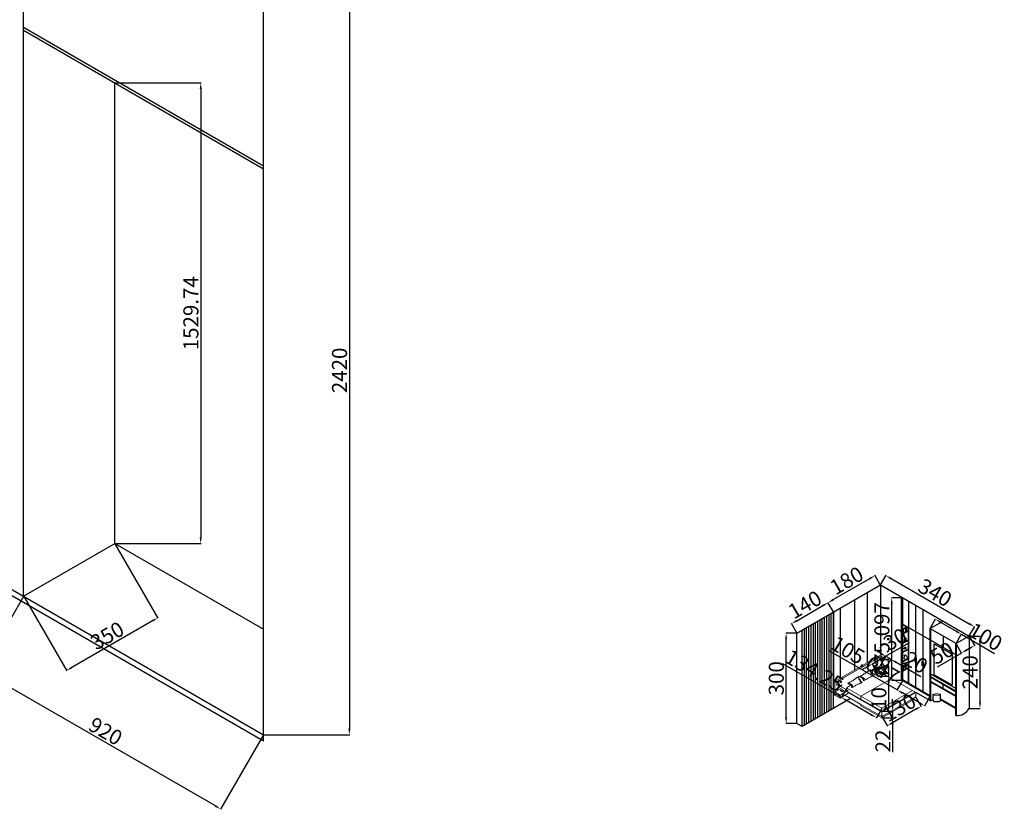
# Model space of a CAD drawing. Units: centimetres. Extents: x 209356 to 217348, y 253987 to 259034.
# Tile 6 of 7: x 214078 to 217348, y 254619 to 257241. Entities that reach past the tile are written whole.
import ezdxf

# ---------------------------------------------------------------- set-up
doc = ezdxf.new("R2010")
doc.units = ezdxf.units.CM
for name, color, linetype, lineweight in [('A-ANNO-DIMS', 2, 'Continuous', 18), ('A-ELEV', 7, 'Continuous', 25), ('A-FURN', 8, 'Continuous', 18)]:
    doc.layers.add(name, color=color, linetype=linetype, lineweight=lineweight)
doc.styles.get("Standard").update_dxf_attribs({"font": 'arial.ttf'})
doc.dimstyles.new('ISO-25', dxfattribs={"dimtxt": 50, "dimasz": 20, "dimexe": 1.25, "dimexo": 0.625, "dimtad": 1, "dimdec": 1, "dimtxsty": 'Standard', "dimcen": 2.5, "dimadec": 0, "dimazin": 0, "dimtfac": 1, "dimtdec": 1, "dimtmove": 0, "dimatfit": 3, "dimfxl": 1, "dimarcsym": 0})

# ---------------------------------------------------------------- blocks, each defined once
blk = doc.blocks.new('BED')
for p, q in [((217490, 254381.4), (217645.9, 254471.4)), ((217494.4, 254378.9), (217650.2, 254468.9)), ((217650.2, 254468.9), (217645.9, 254471.4)), ((217650.2, 254468.9), (217650.2, 254433.8)), ((217619.9, 254421.3), (217645.9, 254436.3)), ((217637.2, 254411.3), (217619.9, 254421.3)), ((217619.9, 254421.3), (217619.9, 254411.3)), ((217637.2, 254401.3), (217619.9, 254411.3)), ((217623.4, 254433.4), (217628.8, 254436.6)), ((217623.4, 254430.2), (217623.4, 254433.4)), ((217623.4, 254430.2), (217628.8, 254433.4)), ((217628.8, 254436.6), (217628.8, 254433.4)), ((217630.5, 254437.7), (217636, 254440.8)), ((217630.5, 254434.5), (217630.5, 254437.7)), ((217630.5, 254434.5), (217636, 254437.6)), ((217631.5, 254423.4), (217637.4, 254426.8)), ((217638.6, 254420.1), (217631.5, 254423.4)), ((217636, 254440.8), (217636, 254437.6)), ((217637.2, 254411.3), (217663.2, 254426.3)), ((217663.2, 254416.3), (217637.2, 254401.3)), ((217637.2, 254411.3), (217637.2, 254401.3)), ((217637.4, 254426.8), (217643.8, 254423.1)), ((217643.8, 254423.1), (217638.6, 254420.1)), ((217642.5, 254427.6), (217641.6, 254424.4)), ((217642.4, 254423.9), (217645.6, 254425.8)), ((217645.6, 254425.8), (217642.5, 254427.6)), ((217645.9, 254436.3), (217663.2, 254426.3)), ((217763, 254347.7), (217653.8, 254410.8)), ((217663.2, 254426.3), (217663.2, 254416.3)), ((217490, 254341.4), (217490, 254381.4)), ((217490, 254381.4), (217494.4, 254378.9)), ((217494.4, 254378.9), (217494.4, 254338.9)), ((217505.5, 254383.3), (217501.1, 254380.8)), ((217501.1, 254380.8), (217501.1, 254370.1)), ((217505.5, 254372.6), (217505.5, 254383.3)), ((217683.4, 254393.7), (217581.2, 254334.7)), ((217494.4, 254348.9), (217520.3, 254363.9)), ((217511.7, 254338.9), (217494.4, 254348.9)), ((217501.1, 254370.1), (217505.5, 254372.6)), ((217504.8, 254365), (217510.2, 254368.1)), ((217504.8, 254361.8), (217504.8, 254365)), ((217504.8, 254361.8), (217510.2, 254364.9)), ((217510.2, 254368.1), (217510.2, 254364.9)), ((217511.7, 254338.9), (217537.7, 254353.9)), ((217511.9, 254369.2), (217517.4, 254372.4)), ((217511.9, 254366), (217511.9, 254369.2)), ((217511.9, 254366), (217517.4, 254369.2)), ((217512.1, 254354), (217517.6, 254357.2)), ((217519.3, 254349.8), (217512.1, 254354)), ((217513.4, 254354), (217513.7, 254354.1)), ((217519.4, 254350.5), (217513.4, 254354)), ((217513.7, 254354.1), (217519.6, 254350.7)), ((217517.4, 254372.4), (217517.4, 254369.2)), ((217517.6, 254357.2), (217524.8, 254353)), ((217524.8, 254353), (217519.3, 254349.8)), ((217519.6, 254350.7), (217519.4, 254350.5)), ((217520.3, 254363.9), (217537.7, 254353.9)), ((217650.5, 254294.7), (217534.2, 254361.9)), ((217534.2, 254361.9), (217534.2, 254355.9)), ((217537.7, 254353.9), (217537.7, 254343.9)), ((217650.5, 254284.7), (217537.7, 254349.9)), ((217650.5, 254282.7), (217537.7, 254347.9)), ((217650.5, 254294.7), (217752.6, 254353.7)), ((217650.5, 254294.7), (217752.6, 254353.7)), ((217650.5, 254284.7), (217761.3, 254348.7)), ((217650.5, 254282.7), (217763, 254347.7)), ((217763, 254347.7), (217763, 254332.7)), ((217494.4, 254338.9), (217490, 254341.4)), ((217494.4, 254338.9), (217511.7, 254328.9)), ((217511.6, 254328.9), (217511.6, 254338.9)), ((217511.6, 254328.9), (217511.6, 254338.9)), ((217537.7, 254343.9), (217511.7, 254328.9)), ((217511.8, 254328.9), (217511.8, 254338.9)), ((217511.8, 254328.9), (217511.8, 254338.9)), ((217581.2, 254307.7), (217528.1, 254338.4)), ((217581.2, 254334.7), (217581.2, 254324.7)), ((217650.5, 254267.7), (217754.4, 254327.7)), ((217650.5, 254262.7), (217754.4, 254322.7)), ((217763, 254332.7), (217754.4, 254327.7)), ((217754.4, 254327.7), (217754.4, 254322.7)), ((217581.2, 254307.7), (217581.2, 254302.7)), ((217581.2, 254307.7), (217650.5, 254267.7)), ((217581.2, 254302.7), (217650.5, 254262.7)), ((217650.5, 254267.7), (217650.5, 254282.7)), ((217650.5, 254262.7), (217650.5, 254267.7))]:
    blk.add_line(p, q)
for centre, radius, start, end in [((217511.1, 254383), 4.19, 39.5108, 167.9055), ((217509.9, 254382.2), 3.31, 44.4187, 149.5181), ((217512.5, 254386.5), 1.96, 260.7432, 336.3872), ((217546.5, 254386.6), 34.4, 183.3938, 192.5417), ((217510.6, 254389.2), 10.4, 283.063, 314.7862), ((217508.4, 254376.4), 11, 29.5129, 57.1752), ((217598, 254351.6), 42.5, 95.8915, 100.3948), ((217568.2, 254330.2), 46.5, 116.4038, 137.0978), ((217559, 254329.1), 42.5, 95.8915, 100.3948)]:
    blk.add_arc(centre, radius, start, end)
for points, knots in [([(217613.5, 254423), (217612.6, 254422.6), (217611.1, 254421.9), (217610.9, 254419.3), (217608.8, 254419.2), (217607.1, 254419.3), (217605.6, 254418.9), (217604.7, 254417.7), (217604.2, 254416.9), (217603.4, 254416.6), (217602.5, 254416.5), (217601.4, 254416.4), (217601, 254415.5), (217600.6, 254414.7), (217599.2, 254413.7), (217597.8, 254413.2), (217596.8, 254412.5), (217595.9, 254411.6), (217595.5, 254410.1), (217593.6, 254408.4), (217591.6, 254409.2), (217589.4, 254408.6), (217589.5, 254407.4), (217588.4, 254404.8), (217584.3, 254405.8), (217582.9, 254403.3), (217581.5, 254403.1), (217580.5, 254402.1), (217579.5, 254401.2), (217578.4, 254400.8), (217577.4, 254400.4), (217576.9, 254400.3), (217576.7, 254400.3)], [0, 0, 0, 0, 2.89084, 4.388481, 6.826027, 7.721705, 9.745954, 11.196809, 12.015907, 12.504109, 13.734618, 14.995994, 15.138853, 16.488821, 17.85858, 20.005577, 20.965006, 21.417944, 23.887049, 25.338073, 28.411278, 29.874196, 30.852713, 31.683987, 37.996546, 38.457682, 40.088873, 41.728901, 42.638341, 43.983164, 45.400565, 45.726572, 45.726572, 45.726572, 45.726572]), ([(217622.9, 254403.5), (217622.4, 254403.9), (217620.8, 254405.3), (217617.3, 254406.2), (217617.4, 254409.5), (217616.4, 254411.4), (217614.8, 254412.2), (217613.4, 254413.1), (217613.1, 254415.9), (217612.2, 254418.7), (217612.1, 254421.4), (217612.1, 254422.3)], [0, 0, 0, 0, 2.032271, 7.025532, 9.57615, 11.808802, 13.736286, 15.379766, 16.848942, 22.474056, 25.423576, 25.423576, 25.423576, 25.423576]), ([(217624.3, 254403.8), (217623.8, 254404.2), (217622.2, 254405.6), (217618.7, 254406.6), (217618.8, 254409.8), (217617.8, 254411.7), (217616.2, 254412.5), (217614.8, 254413.5), (217614.5, 254416.2), (217613.6, 254419.2), (217613.5, 254422), (217613.5, 254423)], [0, 0, 0, 0, 1.85614, 6.416647, 8.746209, 10.785363, 12.545798, 14.046841, 15.388688, 20.526287, 23.621862, 23.621862, 23.621862, 23.621862]), ([(217574.6, 254400.6), (217573.6, 254400.1), (217572.2, 254399.4), (217572, 254396.8), (217569.9, 254396.8), (217568.2, 254396.8), (217566.6, 254396.4), (217565.7, 254395.3), (217565.3, 254394.4), (217564.4, 254394.1), (217563.5, 254394.1), (217562.5, 254393.9), (217562.1, 254393), (217561.6, 254392.2), (217560.3, 254391.2), (217558.8, 254390.7), (217557.9, 254390), (217556.9, 254389.1), (217556.5, 254387.7), (217554.7, 254385.9), (217552.7, 254386.7), (217550.5, 254386.1), (217550.5, 254384.9), (217549.4, 254382.3), (217545.3, 254383.4), (217544, 254380.8), (217542.5, 254380.6), (217541.6, 254379.6), (217540.6, 254378.7), (217539.4, 254378.3), (217538.5, 254377.9), (217537.9, 254377.8), (217537.8, 254377.8)], [0, 0, 0, 0, 2.89084, 4.388481, 6.826027, 7.721705, 9.745954, 11.196809, 12.015907, 12.504109, 13.734618, 14.995994, 15.138853, 16.488821, 17.85858, 20.005577, 20.965006, 21.417944, 23.887049, 25.338073, 28.411278, 29.874196, 30.852713, 31.683987, 37.996546, 38.457682, 40.088873, 41.728901, 42.638341, 43.983164, 45.400565, 45.726572, 45.726572, 45.726572, 45.726572]), ([(217537.8, 254377.8), (217538.7, 254377.4), (217540.5, 254376.7), (217541.7, 254375.3), (217542.3, 254374.6)], [0, 0, 0, 0, 2.919856, 5.565103, 5.565103, 5.565103, 5.565103]), ([(217550.8, 254363), (217551.5, 254364.1), (217552.4, 254365.7), (217554.8, 254365.1), (217555.9, 254367.7), (217560.3, 254367.3), (217564.9, 254373.3), (217572, 254373.8), (217576.8, 254377.2), (217579.5, 254378.8), (217582.7, 254379.5), (217584.5, 254380.8), (217585.3, 254381.4)], [0, 0, 0, 0, 3.455625, 4.661789, 6.322906, 10.419273, 15.636858, 27.307013, 30.016418, 33.147746, 36.597342, 39.668724, 39.668724, 39.668724, 39.668724]), ([(217583.9, 254381), (217583.4, 254381.4), (217581.8, 254382.8), (217578.4, 254383.7), (217578.4, 254387), (217577.4, 254388.9), (217575.8, 254389.7), (217574.4, 254390.6), (217574.2, 254393.4), (217573.3, 254396.3), (217573.2, 254398.9), (217573.2, 254399.8)], [0, 0, 0, 0, 2.032271, 7.025532, 9.57615, 11.808802, 13.736286, 15.379766, 16.848942, 22.474056, 25.423576, 25.423576, 25.423576, 25.423576]), ([(217585.3, 254381.4), (217584.8, 254381.8), (217583.2, 254383.1), (217579.8, 254384.1), (217579.8, 254387.3), (217578.8, 254389.3), (217577.2, 254390.1), (217575.9, 254391), (217575.6, 254393.8), (217574.6, 254396.7), (217574.6, 254399.5), (217574.6, 254400.6)], [0, 0, 0, 0, 1.85614, 6.416647, 8.746209, 10.785363, 12.545798, 14.046841, 15.388688, 20.526287, 23.621862, 23.621862, 23.621862, 23.621862]), ([(217576.7, 254400.3), (217577.7, 254399.9), (217579.4, 254399.2), (217580.7, 254397.8), (217581.3, 254397.1)], [0, 0, 0, 0, 2.919856, 5.565103, 5.565103, 5.565103, 5.565103]), ([(217579.4, 254401.2), (217583.9, 254398.4), (217585.4, 254397.3), (217588.1, 254396.8), (217588.9, 254395), (217590.6, 254393.6), (217590.2, 254391.3), (217591.4, 254389.5), (217591.4, 254388.1), (217591.3, 254387.6)], [0, 0, 0, 0, 4.387716, 5.926297, 8.660034, 10.322113, 12.562773, 15.484437, 17.13725, 17.13725, 17.13725, 17.13725]), ([(217583.9, 254381), (217583.5, 254380.9), (217582.9, 254380.8), (217582.2, 254380.2), (217582.3, 254379.5), (217581.5, 254379.3), (217580.9, 254379.5), (217580.5, 254379.8), (217580.4, 254379.9)], [0, 0, 0, 0, 1.270423, 1.733352, 2.607027, 2.728874, 4.013183, 4.384486, 4.384486, 4.384486, 4.384486]), ([(217581.3, 254397.1), (217582.3, 254396.3), (217583.8, 254395.3), (217586.6, 254394.8), (217587.3, 254392.9), (217589, 254391.6), (217588.6, 254389.3), (217589.8, 254387.4), (217589.8, 254386), (217589.8, 254385.5)], [0, 0, 0, 0, 4.007444, 5.41268, 7.909491, 9.427522, 11.473989, 14.142441, 15.730003, 15.730003, 15.730003, 15.730003]), ([(217589.8, 254385.5), (217590.4, 254386.6), (217591.3, 254388.2), (217593.7, 254387.6), (217594.9, 254390.2), (217599.2, 254389.8), (217603.8, 254395.8), (217611, 254396.3), (217615.7, 254399.7), (217618.4, 254401.3), (217621.6, 254402), (217623.4, 254403.2), (217624.3, 254403.8)], [0, 0, 0, 0, 3.455625, 4.661789, 6.322906, 10.419273, 15.636858, 27.307013, 30.016418, 33.147746, 36.597342, 39.668724, 39.668724, 39.668724, 39.668724]), ([(217622.9, 254403.5), (217622.4, 254403.4), (217621.9, 254403.2), (217621.1, 254402.7), (217621.2, 254402), (217620.5, 254401.8), (217619.8, 254402), (217619.4, 254402.3), (217619.3, 254402.4)], [0, 0, 0, 0, 1.270423, 1.733352, 2.607027, 2.728874, 4.013183, 4.384486, 4.384486, 4.384486, 4.384486]), ([(217542.3, 254374.6), (217543.4, 254373.8), (217544.9, 254372.8), (217547.6, 254372.3), (217548.3, 254370.4), (217550, 254369.1), (217549.7, 254366.8), (217550.9, 254364.9), (217550.8, 254363.5), (217550.8, 254363)], [0, 0, 0, 0, 4.007444, 5.41268, 7.909491, 9.427522, 11.473989, 14.142441, 15.730003, 15.730003, 15.730003, 15.730003]), ([(217543.9, 254376.7), (217545, 254375.9), (217546.4, 254374.8), (217549.2, 254374.3), (217549.9, 254372.5), (217551.6, 254371.1), (217551.2, 254368.8), (217552.4, 254367), (217552.4, 254365.6), (217552.4, 254365.1)], [0, 0, 0, 0, 4.387716, 5.926297, 8.660034, 10.322113, 12.562773, 15.484437, 17.13725, 17.13725, 17.13725, 17.13725])]:
    blk.add_open_spline(points, degree=3, knots=knots)
blk = doc.blocks.new('*D11')
at = {"layer": 'A-ANNO-DIMS', "color": 0, "lineweight": -2, "transparency": 16777216}
for p, q in [((214888.3, 257286.5), (215173.9, 257286.5)), ((215172.6, 257266.5), (215172.6, 254886.5)), ((214888.3, 254866.5), (215173.9, 254866.5))]:
    blk.add_line(p, q, dxfattribs=at)
at = {"layer": 'A-ANNO-DIMS', "color": 0, "transparency": 16777216}
for points in [[(215169.3, 257266.5), (215176, 257266.5), (215172.6, 257286.5)], [(215169.3, 254886.5), (215176, 254886.5), (215172.6, 254866.5)]]:
    blk.add_solid(points, dxfattribs=at)
at = {"layer": 'Defpoints', "color": 0, "transparency": 16777216}
for p in [(214887.6, 257286.5), (214887.6, 254866.5), (215172.6, 254866.5)]:
    blk.add_point(p, dxfattribs=at)
at = {"layer": 'A-ANNO-DIMS', "color": 0, "transparency": 16777216, "insert": (215146.5, 256076.5), "char_height": 50, "attachment_point": 5, "rotation": 90}
blk.add_mtext('2420', dxfattribs=at)
blk = doc.blocks.new('*D27')
at = {"layer": 'A-ANNO-DIMS', "color": 0, "lineweight": -2, "transparency": 16777216}
for p, q in [((214090.6, 255326), (213947.8, 255078.6)), ((214727.8, 254629.7), (213965.7, 255069.7)), ((214887.3, 254866), (214744.5, 254618.6))]:
    blk.add_line(p, q, dxfattribs=at)
at = {"layer": 'A-ANNO-DIMS', "color": 0, "transparency": 16777216}
for points in [[(213967.4, 255072.6), (213964.1, 255066.8), (213948.4, 255079.7)], [(214729.5, 254632.6), (214726.2, 254626.8), (214745.1, 254619.7)]]:
    blk.add_solid(points, dxfattribs=at)
at = {"layer": 'Defpoints', "color": 0, "transparency": 16777216}
for p in [(214090.9, 255326.5), (213948.4, 255079.7), (214887.6, 254866.5)]:
    blk.add_point(p, dxfattribs=at)
at = {"layer": 'A-ANNO-DIMS', "color": 0, "transparency": 16777216, "insert": (214359.9, 254872.4), "char_height": 50, "attachment_point": 5, "rotation": 330}
blk.add_mtext('920', dxfattribs=at)
blk = doc.blocks.new('*D28')
at = {"layer": 'A-ANNO-DIMS', "color": 0, "lineweight": -2, "transparency": 16777216}
for p, q in [((214394.3, 255501), (214537.1, 255253.6)), ((214091.2, 255326), (214234, 255078.6)), ((214519.2, 255244.7), (214250.7, 255089.7))]:
    blk.add_line(p, q, dxfattribs=at)
at = {"layer": 'A-ANNO-DIMS', "color": 0, "transparency": 16777216}
for points in [[(214517.5, 255247.6), (214520.9, 255241.8), (214536.5, 255254.7)], [(214249.1, 255092.6), (214252.4, 255086.8), (214233.4, 255079.7)]]:
    blk.add_solid(points, dxfattribs=at)
at = {"layer": 'Defpoints', "color": 0, "transparency": 16777216}
for p in [(214394, 255501.5), (214090.9, 255326.5), (214233.4, 255079.7)]:
    blk.add_point(p, dxfattribs=at)
at = {"layer": 'A-ANNO-DIMS', "color": 0, "transparency": 16777216, "insert": (214371.9, 255189.9), "char_height": 50, "attachment_point": 5, "rotation": 30}
blk.add_mtext('350', dxfattribs=at)
blk = doc.blocks.new('*D29')
at = {"layer": 'A-ANNO-DIMS', "color": 0, "lineweight": -2, "transparency": 16777216}
for p, q in [((214394.6, 257031.3), (214680.3, 257031.3)), ((214679, 257011.3), (214679, 255521.5)), ((214394.6, 255501.5), (214680.3, 255501.5))]:
    blk.add_line(p, q, dxfattribs=at)
at = {"layer": 'A-ANNO-DIMS', "color": 0, "transparency": 16777216}
for points in [[(214675.7, 257011.3), (214682.3, 257011.3), (214679, 257031.3)], [(214675.7, 255521.5), (214682.3, 255521.5), (214679, 255501.5)]]:
    blk.add_solid(points, dxfattribs=at)
at = {"layer": 'Defpoints', "color": 0, "transparency": 16777216}
for p in [(214394, 257031.3), (214394, 255501.5), (214679, 255501.5)]:
    blk.add_point(p, dxfattribs=at)
at = {"layer": 'A-ANNO-DIMS', "color": 0, "transparency": 16777216, "insert": (214652.9, 256266.4), "char_height": 50, "attachment_point": 5, "rotation": 90}
blk.add_mtext('1529.74', dxfattribs=at)
blk = doc.blocks.new('*D39')
at = {"layer": 'A-ANNO-DIMS', "color": 0, "lineweight": -2, "transparency": 16777216}
for p, q in [((216658.4, 255203.9), (216621.8, 255203.9)), ((216623, 254923.9), (216623, 255183.9)), ((216658.4, 254903.9), (216621.8, 254903.9))]:
    blk.add_line(p, q, dxfattribs=at)
at = {"layer": 'A-ANNO-DIMS', "color": 0, "transparency": 16777216}
for points in [[(216619.7, 255183.9), (216626.4, 255183.9), (216623, 255203.9)], [(216619.7, 254923.9), (216626.4, 254923.9), (216623, 254903.9)]]:
    blk.add_solid(points, dxfattribs=at)
at = {"layer": 'Defpoints', "color": 0, "transparency": 16777216}
for p in [(216623, 255203.9), (216659, 255203.9), (216659, 254903.9)]:
    blk.add_point(p, dxfattribs=at)
at = {"layer": 'A-ANNO-DIMS', "color": 0, "transparency": 16777216, "insert": (216596.9, 255053.9), "char_height": 50, "attachment_point": 5, "rotation": 90}
blk.add_mtext('300', dxfattribs=at)
blk = doc.blocks.new('*D40')
at = {"layer": 'A-ANNO-DIMS', "color": 0, "lineweight": -2, "transparency": 16777216}
for p, q in [((216658.3, 255245.1), (216744.9, 255295.1)), ((216780, 255274.4), (216761.6, 255306.1)), ((216658.7, 255204.4), (216640.4, 255236.1))]:
    blk.add_line(p, q, dxfattribs=at)
at = {"layer": 'A-ANNO-DIMS', "color": 0, "transparency": 16777216}
for points in [[(216743.3, 255297.9), (216746.6, 255292.2), (216762.3, 255305.1)], [(216656.7, 255247.9), (216660, 255242.2), (216641, 255235.1)]]:
    blk.add_solid(points, dxfattribs=at)
at = {"layer": 'Defpoints', "color": 0, "transparency": 16777216}
for p in [(216762.3, 255305.1), (216780.3, 255273.9), (216659, 255203.9)]:
    blk.add_point(p, dxfattribs=at)
at = {"layer": 'A-ANNO-DIMS', "color": 0, "transparency": 16777216, "insert": (216688.6, 255292.7), "char_height": 50, "attachment_point": 5, "rotation": 30}
blk.add_mtext('140', dxfattribs=at)
blk = doc.blocks.new('*D41')
at = {"layer": 'A-ANNO-DIMS', "color": 0, "lineweight": -2, "transparency": 16777216}
for p, q in [((216935.8, 255364.4), (216917.5, 255396.1)), ((216779.6, 255315.1), (216900.8, 255385.1)), ((216780, 255274.4), (216761.6, 255306.1))]:
    blk.add_line(p, q, dxfattribs=at)
at = {"layer": 'A-ANNO-DIMS', "color": 0, "transparency": 16777216}
for points in [[(216899.2, 255387.9), (216902.5, 255382.2), (216918.2, 255395.1)], [(216777.9, 255317.9), (216781.3, 255312.2), (216762.3, 255305.1)]]:
    blk.add_solid(points, dxfattribs=at)
at = {"layer": 'Defpoints', "color": 0, "transparency": 16777216}
for p in [(216918.2, 255395.1), (216936.2, 255363.9), (216780.3, 255273.9)]:
    blk.add_point(p, dxfattribs=at)
at = {"layer": 'A-ANNO-DIMS', "color": 0, "transparency": 16777216, "insert": (216827.1, 255372.7), "char_height": 50, "attachment_point": 5, "rotation": 30}
blk.add_mtext('180', dxfattribs=at)
blk = doc.blocks.new('*D42')
at = {"layer": 'A-ANNO-DIMS', "color": 0, "lineweight": -2, "transparency": 16777216}
for p, q in [((216936.5, 255364.4), (216954.8, 255396.1)), ((216971.5, 255385.1), (217231.3, 255235.1)), ((217230.9, 255194.4), (217249.2, 255226.1))]:
    blk.add_line(p, q, dxfattribs=at)
at = {"layer": 'A-ANNO-DIMS', "color": 0, "transparency": 16777216}
for points in [[(216973.1, 255387.9), (216969.8, 255382.2), (216954.2, 255395.1)], [(217232.9, 255237.9), (217229.6, 255232.2), (217248.6, 255225.1)]]:
    blk.add_solid(points, dxfattribs=at)
at = {"layer": 'Defpoints', "color": 0, "transparency": 16777216}
for p in [(216936.2, 255363.9), (217248.6, 255225.1), (217230.6, 255193.9)]:
    blk.add_point(p, dxfattribs=at)
at = {"layer": 'A-ANNO-DIMS', "color": 0, "transparency": 16777216, "insert": (217114.5, 255332.7), "char_height": 50, "attachment_point": 5, "rotation": 330}
blk.add_mtext('340', dxfattribs=at)
blk = doc.blocks.new('*D43')
at = {"layer": 'A-ANNO-DIMS', "color": 0, "lineweight": -2, "transparency": 16777216}
for p, q in [((217231.2, 255193.9), (217267.9, 255193.9)), ((217266.6, 255173.9), (217266.6, 254973.9)), ((217231.2, 254953.9), (217267.9, 254953.9))]:
    blk.add_line(p, q, dxfattribs=at)
at = {"layer": 'A-ANNO-DIMS', "color": 0, "transparency": 16777216}
for points in [[(217263.3, 255173.9), (217269.9, 255173.9), (217266.6, 255193.9)], [(217263.3, 254973.9), (217269.9, 254973.9), (217266.6, 254953.9)]]:
    blk.add_solid(points, dxfattribs=at)
at = {"layer": 'Defpoints', "color": 0, "transparency": 16777216}
for p in [(217230.6, 255193.9), (217230.6, 254953.9), (217266.6, 254953.9)]:
    blk.add_point(p, dxfattribs=at)
at = {"layer": 'A-ANNO-DIMS', "color": 0, "transparency": 16777216, "insert": (217240.4, 255073.9), "char_height": 50, "attachment_point": 5, "rotation": 90}
blk.add_mtext('240', dxfattribs=at)
blk = doc.blocks.new('*D44')
at = {"layer": 'A-ANNO-DIMS', "color": 0, "lineweight": -2, "transparency": 16777216}
for p, q in [((217101, 255219.4), (217119.3, 255251.1)), ((217136, 255240.1), (217188, 255210.1)), ((217187.6, 255169.4), (217205.9, 255201.1)), ((217205.3, 255200.1), (217315.2, 255136.6))]:
    blk.add_line(p, q, dxfattribs=at)
at = {"layer": 'A-ANNO-DIMS', "color": 0, "transparency": 16777216}
for points in [[(217137.7, 255242.9), (217134.4, 255237.2), (217118.7, 255250.1)], [(217189.6, 255212.9), (217186.3, 255207.2), (217205.3, 255200.1)]]:
    blk.add_solid(points, dxfattribs=at)
at = {"layer": 'Defpoints', "color": 0, "transparency": 16777216}
for p in [(217100.7, 255218.9), (217205.3, 255200.1), (217187.3, 255168.9)]:
    blk.add_point(p, dxfattribs=at)
at = {"layer": 'A-ANNO-DIMS', "color": 0, "transparency": 16777216, "insert": (217282, 255186), "char_height": 50, "attachment_point": 5, "rotation": 330}
blk.add_mtext('100', dxfattribs=at)
blk = doc.blocks.new('*D45')
at = {"layer": 'A-ANNO-DIMS', "color": 0, "lineweight": -2, "transparency": 16777216}
for p, q in [((217187.6, 255168.3), (217205.9, 255136.6)), ((217230.9, 255193.3), (217249.2, 255161.6)), ((217205.3, 255137.7), (217125, 255091.3)), ((217231.3, 255152.7), (217222.6, 255147.7))]:
    blk.add_line(p, q, dxfattribs=at)
at = {"layer": 'A-ANNO-DIMS', "color": 0, "transparency": 16777216}
for points in [[(217229.6, 255155.6), (217232.9, 255149.8), (217248.6, 255162.7)], [(217221, 255150.6), (217224.3, 255144.8), (217205.3, 255137.7)]]:
    blk.add_solid(points, dxfattribs=at)
at = {"layer": 'Defpoints', "color": 0, "transparency": 16777216}
for p in [(217187.3, 255168.9), (217230.6, 255193.9), (217205.3, 255137.7)]:
    blk.add_point(p, dxfattribs=at)
at = {"layer": 'A-ANNO-DIMS', "color": 0, "transparency": 16777216, "insert": (217143.4, 255132.2), "char_height": 50, "attachment_point": 5, "rotation": 30}
blk.add_mtext('50', dxfattribs=at)
blk = doc.blocks.new('*D46')
at = {"layer": 'A-ANNO-DIMS', "color": 0, "lineweight": -2, "transparency": 16777216}
for p, q in [((217009.1, 255321.3), (216972.5, 255321.3)), ((216973.7, 255066.2), (216973.7, 255301.3)), ((217009.1, 255046.2), (216972.5, 255046.2))]:
    blk.add_line(p, q, dxfattribs=at)
at = {"layer": 'A-ANNO-DIMS', "color": 0, "transparency": 16777216}
for points in [[(216970.4, 255301.3), (216977.1, 255301.3), (216973.7, 255321.3)], [(216970.4, 255066.2), (216977.1, 255066.2), (216973.7, 255046.2)]]:
    blk.add_solid(points, dxfattribs=at)
at = {"layer": 'Defpoints', "color": 0, "transparency": 16777216}
for p in [(216973.7, 255321.3), (217009.7, 255321.3), (217009.7, 255046.2)]:
    blk.add_point(p, dxfattribs=at)
at = {"layer": 'A-ANNO-DIMS', "color": 0, "transparency": 16777216, "insert": (216947.6, 255183.8), "char_height": 50, "attachment_point": 5, "rotation": 90}
blk.add_mtext('275.097', dxfattribs=at)
blk = doc.blocks.new('*D47')
at = {"layer": 'A-ANNO-DIMS', "color": 0, "lineweight": -2, "transparency": 16777216}
for p, q in [((216991.7, 255015), (216764, 255146.5)), ((217009.4, 255045.7), (216991.1, 255013.9)), ((217065.4, 254972.5), (217009, 255005)), ((217100.4, 254993.1), (217082.1, 254961.4))]:
    blk.add_line(p, q, dxfattribs=at)
at = {"layer": 'A-ANNO-DIMS', "color": 0, "transparency": 16777216}
for points in [[(217010.7, 255007.9), (217007.4, 255002.1), (216991.7, 255015)], [(217067, 254975.4), (217063.7, 254969.6), (217082.7, 254962.5)]]:
    blk.add_solid(points, dxfattribs=at)
at = {"layer": 'Defpoints', "color": 0, "transparency": 16777216}
for p in [(217009.7, 255046.2), (216991.7, 255015), (217100.7, 254993.7)]:
    blk.add_point(p, dxfattribs=at)
at = {"layer": 'A-ANNO-DIMS', "color": 0, "transparency": 16777216, "insert": (216882.3, 255108.4), "char_height": 50, "attachment_point": 5, "rotation": 330}
blk.add_mtext('105.047', dxfattribs=at)
blk = doc.blocks.new('*D48')
at = {"layer": 'A-ANNO-DIMS', "color": 0, "lineweight": -2, "transparency": 16777216}
for p, q in [((217053.6, 254991.6), (217071.9, 254959.9)), ((217054, 254951), (216976, 254906)), ((216941, 254926.6), (216959.3, 254894.9))]:
    blk.add_line(p, q, dxfattribs=at)
at = {"layer": 'A-ANNO-DIMS', "color": 0, "transparency": 16777216}
for points in [[(217052.3, 254953.9), (217055.6, 254948.1), (217071.3, 254961)], [(216974.4, 254908.9), (216977.7, 254903.1), (216958.7, 254896)]]:
    blk.add_solid(points, dxfattribs=at)
at = {"layer": 'Defpoints', "color": 0, "transparency": 16777216}
for p in [(217053.3, 254992.2), (216940.7, 254927.2), (216958.7, 254896)]:
    blk.add_point(p, dxfattribs=at)
at = {"layer": 'A-ANNO-DIMS', "color": 0, "transparency": 16777216, "insert": (217001.9, 254951.1), "char_height": 50, "attachment_point": 5, "rotation": 30}
blk.add_mtext('130', dxfattribs=at)
blk = doc.blocks.new('*D49')
at = {"layer": 'A-ANNO-DIMS', "color": 0, "lineweight": -2, "transparency": 16777216}
for p, q in [((216806.4, 254990.1), (216612, 255102.3)), ((216824.1, 255020.7), (216805.8, 254989)), ((216905.4, 254933), (216823.8, 254980.1)), ((216940.4, 254953.6), (216922.1, 254921.9))]:
    blk.add_line(p, q, dxfattribs=at)
at = {"layer": 'A-ANNO-DIMS', "color": 0, "transparency": 16777216}
for points in [[(216825.4, 254983), (216822.1, 254977.2), (216806.4, 254990.1)], [(216907, 254935.9), (216903.7, 254930.1), (216922.7, 254923)]]:
    blk.add_solid(points, dxfattribs=at)
at = {"layer": 'Defpoints', "color": 0, "transparency": 16777216}
for p in [(216824.4, 255021.3), (216806.4, 254990.1), (216940.7, 254954.2)]:
    blk.add_point(p, dxfattribs=at)
at = {"layer": 'A-ANNO-DIMS', "color": 0, "transparency": 16777216, "insert": (216713.7, 255073.9), "char_height": 50, "attachment_point": 5, "rotation": 330}
blk.add_mtext('134.25', dxfattribs=at)
blk = doc.blocks.new('*D50')
at = {"layer": 'A-ANNO-DIMS', "color": 0, "lineweight": -2, "transparency": 16777216}
for p, q in [((216976.7, 254964.2), (216976.7, 254984.2)), ((216941.3, 254944.2), (216978, 254944.2)), ((216976.7, 254944.2), (216976.7, 254922.2)), ((216941.3, 254922.2), (216978, 254922.2)), ((216976.7, 254902.2), (216976.7, 254808.9))]:
    blk.add_line(p, q, dxfattribs=at)
at = {"layer": 'A-ANNO-DIMS', "color": 0, "transparency": 16777216}
for points in [[(216973.4, 254964.2), (216980, 254964.2), (216976.7, 254944.2)], [(216973.4, 254902.2), (216980, 254902.2), (216976.7, 254922.2)]]:
    blk.add_solid(points, dxfattribs=at)
at = {"layer": 'Defpoints', "color": 0, "transparency": 16777216}
for p in [(216940.7, 254944.2), (216940.7, 254922.2), (216976.7, 254922.2)]:
    blk.add_point(p, dxfattribs=at)
at = {"layer": 'A-ANNO-DIMS', "color": 0, "transparency": 16777216, "insert": (216951, 254845.5), "char_height": 50, "attachment_point": 5, "rotation": 90}
blk.add_mtext('22', dxfattribs=at)
blk = doc.blocks.new('*D51')
at = {"layer": 'A-ANNO-DIMS', "color": 0, "lineweight": -2, "transparency": 16777216}
for p, q in [((216952.8, 255126.9), (217033, 255173.2)), ((216927.2, 255071.2), (216908.9, 255103)), ((216909.5, 255101.9), (216935.5, 255116.9)), ((216953.2, 255086.2), (216934.8, 255118)), ((216892.2, 255091.9), (216874.9, 255081.9))]:
    blk.add_line(p, q, dxfattribs=at)
at = {"layer": 'A-ANNO-DIMS', "color": 0, "transparency": 16777216}
for points in [[(216951.1, 255129.8), (216954.5, 255124), (216935.5, 255116.9)], [(216890.5, 255094.8), (216893.8, 255089), (216909.5, 255101.9)]]:
    blk.add_solid(points, dxfattribs=at)
at = {"layer": 'Defpoints', "color": 0, "transparency": 16777216}
for p in [(216935.5, 255116.9), (216927.5, 255070.7), (216953.5, 255085.7)]:
    blk.add_point(p, dxfattribs=at)
at = {"layer": 'A-ANNO-DIMS', "color": 0, "transparency": 16777216, "insert": (216988.5, 255177.7), "char_height": 50, "attachment_point": 5, "rotation": 30}
blk.add_mtext('30', dxfattribs=at)
blk = doc.blocks.new('*D52')
at = {"layer": 'A-ANNO-DIMS', "color": 0, "lineweight": -2, "transparency": 16777216}
for p, q in [((216936.8, 255136.9), (216919.5, 255146.9)), ((216936.5, 255096.2), (216954.8, 255128)), ((216953.8, 255086.2), (216972.1, 255118)), ((216954.2, 255126.9), (216971.5, 255116.9)), ((216988.8, 255106.9), (217069.8, 255060.1))]:
    blk.add_line(p, q, dxfattribs=at)
at = {"layer": 'A-ANNO-DIMS', "color": 0, "transparency": 16777216}
for points in [[(216938.5, 255139.8), (216935.2, 255134), (216954.2, 255126.9)], [(216990.5, 255109.8), (216987.1, 255104), (216971.5, 255116.9)]]:
    blk.add_solid(points, dxfattribs=at)
at = {"layer": 'Defpoints', "color": 0, "transparency": 16777216}
for p in [(216971.5, 255116.9), (216936.2, 255095.7), (216953.5, 255085.7)]:
    blk.add_point(p, dxfattribs=at)
at = {"layer": 'A-ANNO-DIMS', "color": 0, "transparency": 16777216, "insert": (217051, 255101.1), "char_height": 50, "attachment_point": 5, "rotation": 330}
blk.add_mtext('20', dxfattribs=at)
blk = doc.blocks.new('*D53')
at = {"layer": 'A-ANNO-DIMS', "color": 0, "lineweight": -2, "transparency": 16777216}
for p, q in [((216963.5, 255090.7), (216963.5, 255110.7)), ((216928.1, 255070.7), (216964.7, 255070.7)), ((216963.5, 255070.7), (216963.5, 255060.7)), ((216928.1, 255060.7), (216964.7, 255060.7)), ((216963.5, 255040.7), (216963.5, 254952.7))]:
    blk.add_line(p, q, dxfattribs=at)
at = {"layer": 'A-ANNO-DIMS', "color": 0, "transparency": 16777216}
for points in [[(216960.2, 255090.7), (216966.8, 255090.7), (216963.5, 255070.7)], [(216960.2, 255040.7), (216966.8, 255040.7), (216963.5, 255060.7)]]:
    blk.add_solid(points, dxfattribs=at)
at = {"layer": 'Defpoints', "color": 0, "transparency": 16777216}
for p in [(216927.5, 255070.7), (216927.5, 255060.7), (216963.5, 255060.7)]:
    blk.add_point(p, dxfattribs=at)
at = {"layer": 'A-ANNO-DIMS', "color": 0, "transparency": 16777216, "insert": (216937.3, 254986.7), "char_height": 50, "attachment_point": 5, "rotation": 90}
blk.add_mtext('10', dxfattribs=at)

msp = doc.modelspace()

# ---------------------------------------------------------------- linework, layer by layer
at = {"layer": 'A-ELEV'}
for p, q in [((214090.9016, 255326.5492), (214090.9016, 257726.5492)), ((214887.645, 254846.5492), (214887.645, 257286.5492)), ((214090.9016, 257216.2903), (214887.645, 256756.2903)), ((214090.9016, 257206.2903), (214887.645, 256746.2903)), ((214394.0105, 255501.5492), (214394.0105, 257031.2903)), ((212289.5688, 256366.5492), (214887.645, 254866.5492)), ((212289.5688, 256346.5492), (214887.645, 254846.5492)), ((214090.9016, 255326.5492), (214090.9016, 256206.5492)), ((214090.9016, 255326.5492), (214394.0105, 255501.5492)), ((214394.0105, 255501.5492), (214887.645, 255216.5492)), ((216659.0263, 255203.8753), (216936.1545, 255363.8753)), ((216936.1545, 255363.8753), (217230.6031, 255193.8753)), ((216936.1545, 255363.8753), (216936.1545, 255130.7786)), ((216891.8587, 255338.3011), (216891.8587, 255105.2044)), ((216849.5484, 255313.8733), (216849.5484, 255080.7765)), ((217005.4365, 255323.8753), (217005.4365, 255048.6859)), ((217009.7261, 255321.3064), (217009.7261, 255234.1262)), ((217029.2522, 255310.1253), (217029.2522, 255222.8528)), ((217053.0679, 255296.3753), (217053.0679, 255023.1859)), ((216758.0007, 254941.0182), (216758.0007, 255261.0182)), ((216758.0007, 254941.0182), (216758.0007, 255261.0182)), ((216758.0007, 254941.0182), (216758.0007, 255261.0182)), ((216765.4238, 254945.3039), (216765.4238, 255265.3039)), ((216765.4238, 254945.3039), (216765.4238, 255265.3039)), ((216772.8468, 254949.5896), (216772.8468, 255269.5896)), ((216772.8468, 254949.5896), (216772.8468, 255269.5896)), ((216780.2699, 255273.8753), (216780.2699, 255040.7786)), ((216780.2699, 254953.8753), (216780.2699, 255273.8753)), ((216780.2699, 255040.7786), (216780.2699, 255273.8753)), ((216802.6023, 255286.7689), (216802.6023, 255053.6722)), ((217076.8836, 255282.6253), (217076.8836, 255009.4359)), ((216706.0392, 254911.0182), (216706.0392, 255231.0182)), ((216706.0392, 254911.0182), (216706.0392, 255231.0182)), ((216713.4622, 254915.3039), (216713.4622, 255235.3039)), ((216713.4622, 254915.3039), (216713.4622, 255235.3039)), ((216713.4622, 255002.4919), (216713.4622, 255235.3039)), ((216713.4622, 255002.4919), (216713.4622, 255235.3039)), ((216720.8853, 254919.5896), (216720.8853, 255239.5896)), ((216720.8853, 254919.5896), (216720.8853, 255239.5896)), ((216720.8853, 255006.7776), (216720.8853, 255239.5896)), ((216720.8853, 255006.7776), (216720.8853, 255239.5896)), ((216728.3084, 254923.8753), (216728.3084, 255243.8753)), ((216728.3084, 254923.8753), (216728.3084, 255243.8753)), ((216728.3084, 255011.0633), (216728.3084, 255243.8753)), ((216728.3084, 255011.0633), (216728.3084, 255243.8753)), ((216735.7315, 254928.161), (216735.7315, 255248.161)), ((216735.7315, 254928.161), (216735.7315, 255248.161)), ((216735.7315, 255015.3491), (216735.7315, 255248.161)), ((216735.7315, 255015.3491), (216735.7315, 255248.161)), ((216743.1545, 254932.4468), (216743.1545, 255252.4468)), ((216743.1545, 254932.4468), (216743.1545, 255252.4468)), ((216743.1545, 255019.6348), (216743.1545, 255252.4468)), ((216743.1545, 255019.6348), (216743.1545, 255252.4468)), ((216750.5776, 254936.7325), (216750.5776, 255256.7325)), ((216750.5776, 255023.9205), (216750.5776, 255256.7325)), ((216750.5776, 255023.9205), (216750.5776, 255256.7325)), ((217100.6993, 255181.6028), (217009.7261, 255234.1262)), ((217009.7261, 255232.1262), (217009.7261, 255046.2093)), ((217029.2522, 255220.8528), (217009.7261, 255232.1262)), ((217100.6993, 255218.8753), (217144.0006, 255243.8753)), ((216659.0263, 254903.8753), (216659.0263, 255203.8753)), ((216659.0263, 254903.8753), (216659.0263, 255203.8753)), ((216676.3469, 254893.8753), (216676.3469, 255213.8753)), ((216676.3469, 254893.8753), (216676.3469, 255213.8753)), ((216683.7699, 254898.161), (216683.7699, 255218.161)), ((216683.7699, 254898.161), (216683.7699, 255218.161)), ((216691.193, 254902.4468), (216691.193, 255222.4468)), ((216691.193, 254902.4468), (216691.193, 255222.4468)), ((216698.6161, 254906.7325), (216698.6161, 255226.7325)), ((216698.6161, 254906.7325), (216698.6161, 255226.7325)), ((217009.7261, 255201.4734), (217028.8192, 255212.4968)), ((217009.7603, 255200.474), (217028.8534, 255211.4974)), ((217013.3153, 255208.7538), (217013.3153, 255218.0479)), ((217018.7961, 255219.701), (217019.1832, 255207.6293)), ((217022.9681, 255223.6209), (217022.9681, 255212.2523)), ((217028.8192, 255221.1028), (217028.8192, 255037.1859)), ((217029.2522, 255220.8528), (217029.2522, 255036.9359)), ((217187.3018, 255168.8753), (217100.6993, 255218.8753)), ((217100.6993, 255218.8753), (217100.6993, 254979.7786)), ((217102.4314, 255217.8753), (217102.4314, 254978.7786)), ((217009.7261, 255170.8206), (217028.8192, 255181.844)), ((217009.8482, 255169.828), (217028.9413, 255180.8514)), ((217015.7269, 255174.9664), (217015.7269, 255184.6044)), ((217185.5698, 255132.6028), (217102.4314, 255180.6028)), ((217114.7876, 255167.8752), (217174.1756, 255133.5875)), ((217114.7876, 255065.7067), (217114.7876, 255167.8752)), ((217144.0006, 255193.8753), (217144.0006, 255156.6028)), ((217185.5698, 255169.8753), (217185.5698, 254930.7786)), ((217230.6031, 255193.8753), (217187.3018, 255168.8753)), ((217187.3018, 255168.8753), (217187.3018, 254929.7786)), ((217230.6031, 255193.8753), (217230.6031, 254953.8753)), ((217009.7261, 255140.1677), (217028.8192, 255151.1911)), ((217009.7655, 255139.1685), (217028.8586, 255150.1919)), ((217174.1756, 255133.5875), (217174.1756, 255031.419)), ((217009.7261, 255109.5149), (217028.8192, 255120.5383)), ((217009.7261, 255108.5149), (217028.8192, 255119.5383)), ((217019.0193, 255085.2671), (217019.0193, 255098.491)), ((217020.3357, 255115.9516), (217022.9555, 255116.8416)), ((217052.1015, 255122.5563), (217049.9324, 255123.8087)), ((217049.9324, 255123.8087), (217049.9324, 255109.8011)), ((217049.9324, 255109.8011), (217052.1015, 255108.8482)), ((217052.1015, 255108.8482), (217052.1015, 255122.5563)), ((217056.2702, 255120.1495), (217054.1012, 255121.4018)), ((217054.1012, 255121.4018), (217054.1012, 255107.3943)), ((217054.1012, 255107.3943), (217056.2702, 255106.4414)), ((217056.2702, 255106.4414), (217056.2702, 255120.1495)), ((217075.8373, 255109.0468), (217073.6682, 255110.2991)), ((217073.6682, 255110.2991), (217073.6682, 255096.2916)), ((217075.8373, 255095.3387), (217075.8373, 255109.0468)), ((217080.2313, 255106.3156), (217078.0623, 255107.5679)), ((217078.0623, 255107.5679), (217078.0623, 255093.5604)), ((217080.2313, 255092.6075), (217080.2313, 255106.3156)), ((217009.7261, 255078.8621), (217028.8192, 255089.8855)), ((217009.7261, 255077.8621), (217028.8192, 255088.8855)), ((217012.7805, 255083.0899), (217012.7805, 255094.889)), ((217073.6682, 255096.2916), (217075.8373, 255095.3387)), ((217078.0623, 255093.5604), (217080.2313, 255092.6075)), ((217102.4314, 255068.5749), (217185.5698, 255020.5749)), ((217174.1756, 255031.419), (217114.7876, 255065.7067)), ((216802.6023, 255043.9361), (216802.6023, 255042.2981)), ((217100.6993, 254993.6859), (217005.4365, 255048.6859)), ((217100.6993, 254995.6859), (217009.7261, 255048.2093)), ((217102.4314, 255060.1615), (217185.5698, 255012.1615)), ((217102.4314, 255058.1615), (217185.5698, 255010.1615)), ((217102.4314, 255044.389), (217185.5698, 254996.389)), ((217102.4314, 255042.389), (217185.5698, 254994.389)), ((217144.0006, 255020.389), (217144.0006, 255034.1615)), ((217102.4314, 254978.7786), (217053.285, 255007.1532)), ((217111.1891, 254981.1472), (217111.1891, 254999.7642)), ((217135.6098, 254981.1472), (217135.6098, 254999.7672)), ((216837.3438, 254986.827), (216676.3469, 254893.8753)), ((217102.4314, 254978.7786), (217111.1891, 254983.8349)), ((217115.1891, 254977.1472), (217131.6098, 254977.1472)), ((217185.5698, 254955.7728), (217135.6098, 254984.6172)), ((217185.5698, 254953.7728), (217135.6098, 254982.6172)), ((216750.5776, 254936.7325), (216750.5776, 254958.9205)), ((216758.0007, 254941.0182), (216758.0007, 254947.0617)), ((216676.3469, 254893.8753), (216659.0263, 254903.8753)), ((217187.3018, 254929.7786), (217185.5698, 254930.7786))]:
    msp.add_line(p, q, dxfattribs=at)
for centre, radius, start, end in [((217017.1936, 255213.1191), 5.8392, 228.3815172, 351.4628974), ((217013.6284, 255090.6874), 7.6447, 263.6317938, 314.8436985), ((217115.1891, 254981.1472), 4, 180, 270), ((217131.6098, 254981.1472), 4, 270, 0), ((217189.2472, 254977.2368), 47.4981, 267.6526665, 330.5383611)]:
    msp.add_arc(centre, radius, start, end, dxfattribs=at)
for p in [(217009.7261, 255201.4734), (217009.7261, 255170.8206), (217009.7261, 255140.1677), (217009.7261, 255109.5149), (217009.7261, 255078.8621)]:
    msp.add_point(p, dxfattribs=at)
at = {"layer": 'A-FURN'}
for centre, major_axis, ratio in [((217018.1417, 255220.8344), (-4.8264, -2.7865), 0.234842156), ((217017.2318, 255130.6005), (2.5708, 0.9377), 0.233310182), ((217015.8999, 255096.69), (3.1194, 1.801), 0.334063547), ((217123.3995, 254999.7657), (-12.2104, 0), 0.216737689)]:
    msp.add_ellipse(centre, major_axis=major_axis, ratio=ratio, dxfattribs=at)
for points, knots in [([(217015.7269, 255184.6044), (217017.3417, 255185.5367), (217019.4883, 255186.776), (217021.6349, 255188.0154), (217022.1667, 255188.3224)], [0, 0, 0, 0, 5.593798204, 7.435984157, 7.435984157, 7.435984157, 7.435984157]), ([(217015.7269, 255174.9664), (217016.4889, 255175.7131), (217017.3949, 255176.6009), (217018.0896, 255177.9805), (217018.3217, 255178.681), (217018.8425, 255179.2829), (217019.6374, 255179.4539), (217020.7485, 255179.7311), (217021.1829, 255180.9794), (217021.9338, 255181.2563), (217022.1667, 255181.3422)], [0, 0, 0, 0, 3.158737294, 3.75561648, 4.610395012, 5.380210726, 5.984402095, 7.018276091, 8.635454641, 9.362166761, 9.362166761, 9.362166761, 9.362166761]), ([(217022.1667, 255188.3224), (217022.1667, 255186.5736), (217022.1667, 255184.2469), (217022.1667, 255181.9202), (217022.1667, 255181.3422)], [0, 0, 0, 0, 5.246246576, 6.980167584, 6.980167584, 6.980167584, 6.980167584]), ([(217013.5915, 255152.4226), (217014.1677, 255153.0134), (217015.1083, 255153.9778), (217016.1965, 255155.6701), (217016.9992, 255156.5403), (217017.4483, 255157.0272)], [0, 0, 0, 0, 2.467711004, 4.02890651, 6.012426458, 6.012426458, 6.012426458, 6.012426458]), ([(217013.5915, 255152.4226), (217014.0146, 255152.2006), (217014.6826, 255151.8499), (217015.6702, 255151.3515), (217016.3882, 255151.6094), (217017.0382, 255151.2837), (217017.4522, 255151.2468), (217017.7663, 255151.2189)], [0, 0, 0, 0, 1.449298222, 2.288532828, 3.187615933, 3.485673989, 4.421683215, 4.421683215, 4.421683215, 4.421683215]), ([(217017.4483, 255157.0272), (217017.9237, 255156.9645), (217018.9309, 255156.8315), (217019.9988, 255155.7205), (217021.0873, 255156.4111), (217021.3555, 255156.0179), (217021.4469, 255155.8838)], [0, 0, 0, 0, 1.431710338, 3.033340857, 3.881301031, 4.320251313, 4.320251313, 4.320251313, 4.320251313]), ([(217017.7663, 255151.2189), (217017.91, 255151.1216), (217018.2239, 255150.9094), (217018.7006, 255151.3046), (217019.134, 255151.329), (217019.507, 255151.2467), (217019.6579, 255151.2117)], [0, 0, 0, 0, 0.47277139, 1.032177412, 1.549347441, 1.891074354, 1.891074354, 1.891074354, 1.891074354]), ([(217021.4469, 255155.8838), (217020.9334, 255154.5427), (217020.4199, 255153.2016), (217019.9064, 255151.8605), (217019.8236, 255151.6442), (217019.7407, 255151.4279), (217019.6579, 255151.2117)], [0, 0, 0, 0, 4.308222762, 4.308222762, 4.308222762, 5.002956576, 5.002956576, 5.002956576, 5.002956576]), ([(217019.6579, 255151.2117), (217020.3502, 255151.5733), (217021.1461, 255151.9891), (217020.773, 255152.8011), (217020.9942, 255153.3021), (217021.2861, 255153.5883), (217021.4725, 255153.7711)], [0, 0, 0, 0, 1.780264413, 2.047013876, 2.49424977, 3.284312932, 3.284312932, 3.284312932, 3.284312932]), ([(217019.8012, 255131.544), (217020.0006, 255130.7245), (217020.2723, 255129.6076), (217021.6431, 255127.6089), (217025.8136, 255126.3801), (217025.4995, 255120.247), (217023.5591, 255117.6495), (217022.9555, 255116.8416)], [0, 0, 0, 0, 2.501508236, 3.409368686, 7.165621256, 13.985591082, 17.064349375, 17.064349375, 17.064349375, 17.064349375]), ([(217021.4469, 255155.8838), (217021.5507, 255155.4854), (217021.694, 255154.9355), (217021.4563, 255154.2493), (217021.467, 255153.9341), (217021.4725, 255153.7711)], [0, 0, 0, 0, 1.19282593, 1.646616743, 2.132281644, 2.132281644, 2.132281644, 2.132281644]), ([(217014.6605, 255129.6639), (217015.0785, 255129.272), (217016.0694, 255128.3429), (217016.3719, 255126.0986), (217014.6511, 255123.7609), (217014.4048, 255119.5272), (217017.6671, 255117.0162), (217019.741, 255116.1889), (217020.3357, 255115.9516)], [0, 0, 0, 0, 1.698128731, 4.025634494, 5.932086627, 10.256929285, 15.073768224, 17.010233929, 17.010233929, 17.010233929, 17.010233929]), ([(217019.0193, 255098.491), (217020.1128, 255099.1284), (217023.2095, 255100.9336), (217022.133, 255091.5201), (217020.2183, 255087.675), (217019.0193, 255085.2671)], [0, 0, 0, 0, 3.044994261, 8.623023804, 17.968671873, 17.968671873, 17.968671873, 17.968671873]), ([(217019.0193, 255097.9742), (217019.7893, 255098.4786), (217022.2717, 255099.5578), (217021.3842, 255091.7975), (217019.9017, 255088.0287), (217019.0193, 255086.1469)], [0.832719008, 0.832719008, 0.832719008, 0.832719008, 3.044994261, 8.623023804, 15.6457898, 15.6457898, 15.6457898, 15.6457898])]:
    msp.add_open_spline(points, degree=3, knots=knots, dxfattribs=at)

# ---------------------------------------------------------------- block references
msp.add_blockref('BED', (-709.7554, 659.4251), dxfattribs=at)

# ---------------------------------------------------------------- dimensions: what is measured, and where the dimension line sits
at = {"layer": 'A-ANNO-DIMS'}
for base, p1, p2, angle, override, picture, middle in [((215172.645, 254866.5492), (214887.645, 257286.5492), (214887.645, 254866.5492), 270, {"dimdec": 0, "dimlfac": 1, "dimrnd": 0, "dimzin": 0, "dimdsep": 46, "dimlunit": 2}, '*D11', (215146.4913, 256076.5492)), ((214679.0105, 255501.5492), (214394.0105, 257031.2903), (214394.0105, 255501.5492), 270, {"dimdec": 2, "dimlfac": 1, "dimrnd": 0, "dimzin": 0, "dimdsep": 46, "dimlunit": 2}, '*D29', (214652.8569, 256266.4197)), ((214233.4016, 255079.7319), (214394.0105, 255501.5492), (214090.9016, 255326.5492), 210, {"dimdec": 0, "dimlfac": 1, "dimrnd": 0, "dimzin": 0, "dimdsep": 46, "dimlunit": 2}, '*D28', (214371.8707, 255189.8964)), ((216918.1545, 255395.0522), (216780.2699, 255273.8753), (216936.1545, 255363.8753), 30, {"dimdec": 0, "dimlfac": 1, "dimrnd": 0, "dimzin": 0, "dimdsep": 46, "dimlunit": 2}, '*D41', (216827.1354, 255372.702)), ((217248.6031, 255225.0522), (216936.1545, 255363.8753), (217230.6031, 255193.8753), 330, {"dimdec": 0, "dimlfac": 1, "dimrnd": 0, "dimzin": 0, "dimdsep": 46, "dimlunit": 2}, '*D42', (217114.4641, 255332.7167)), ((213948.4016, 255079.7319), (214887.645, 254866.5492), (214090.9016, 255326.5492), 150, {"dimdec": 0, "dimlfac": 1, "dimrnd": 0, "dimzin": 0, "dimdsep": 46, "dimlunit": 2}, '*D27', (214359.8501, 254872.3816)), ((216762.2699, 255305.0522), (216659.0263, 255203.8753), (216780.2699, 255273.8753), 30, {"dimdec": 0, "dimlfac": 1, "dimrnd": 0, "dimzin": 0, "dimdsep": 46, "dimlunit": 2}, '*D40', (216688.5713, 255292.702)), ((216973.7261, 255321.3064), (217009.7261, 255046.2093), (217009.7261, 255321.3064), 90, {"dimdec": 3, "dimlfac": 1, "dimrnd": 0, "dimzin": 0, "dimdsep": 46, "dimlunit": 2}, '*D46', (216947.5725, 255183.7578)), ((217205.3018, 255200.0522), (217100.6993, 255218.8753), (217187.3018, 255168.8753), 330, {"dimdec": 0, "dimlfac": 1, "dimrnd": 0, "dimzin": 0, "dimdsep": 46, "dimlunit": 2}, '*D44', (217281.9637, 255185.9911)), ((216623.0263, 255203.8753), (216659.0263, 254903.8753), (216659.0263, 255203.8753), 90, {"dimdec": 0, "dimlfac": 1, "dimrnd": 0, "dimzin": 0, "dimdsep": 46, "dimlunit": 2}, '*D39', (216596.8556, 255053.8753)), ((216991.7261, 255015.0323), (217100.6993, 254993.6859), (217009.7261, 255046.2093), 150, {"dimdec": 3, "dimlfac": 1, "dimrnd": 0, "dimzin": 0, "dimdsep": 46, "dimlunit": 2}, '*D47', (216882.2767, 255108.4226)), ((216935.475, 255116.8803), (216927.4942, 255070.7034), (216953.475, 255085.7034), 30, {"dimdec": 0, "dimlfac": 1, "dimrnd": 0, "dimzin": 0, "dimdsep": 46, "dimlunit": 2}, '*D51', (216988.4972, 255177.712)), ((217205.3018, 255137.6984), (217230.6031, 255193.8753), (217187.3018, 255168.8753), 210, {"dimdec": 0, "dimlfac": 1, "dimrnd": 0, "dimzin": 0, "dimdsep": 46, "dimlunit": 2}, '*D45', (217143.4232, 255132.1724)), ((217266.6031, 254953.8753), (217230.6031, 255193.8753), (217230.6031, 254953.8753), 270, {"dimdec": 0, "dimlfac": 1, "dimrnd": 0, "dimzin": 0, "dimdsep": 46, "dimlunit": 2}, '*D43', (217240.4495, 255073.8753)), ((216806.4372, 254990.1017), (216940.7017, 254954.1532), (216824.4372, 255021.2786), 150, {"dimdec": 2, "dimlfac": 1, "dimrnd": 0, "dimzin": 0, "dimdsep": 46, "dimlunit": 2}, '*D49', (216713.6552, 255073.8887)), ((216971.475, 255116.8803), (216936.1545, 255095.7034), (216953.475, 255085.7034), 330, {"dimdec": 0, "dimlfac": 1, "dimrnd": 0, "dimzin": 0, "dimdsep": 46, "dimlunit": 2}, '*D52', (217051.0433, 255101.1411)), ((216963.4942, 255060.7034), (216927.4942, 255070.7034), (216927.4942, 255060.7034), 270, {"dimdec": 0, "dimlfac": 1, "dimrnd": 0, "dimzin": 0, "dimdsep": 46, "dimlunit": 2}, '*D53', (216937.3406, 254986.7053)), ((216958.7017, 254895.9763), (217053.285, 254992.1532), (216940.7017, 254927.1532), 210, {"dimdec": 0, "dimlfac": 1, "dimrnd": 0, "dimzin": 0, "dimdsep": 46, "dimlunit": 2}, '*D48', (217001.908, 254951.1408)), ((216976.7017, 254922.1532), (216940.7017, 254944.1532), (216940.7017, 254922.1532), 270, {"dimdec": 0, "dimlfac": 1, "dimrnd": 0, "dimzin": 0, "dimdsep": 46, "dimlunit": 2}, '*D50', (216950.9744, 254845.546))]:
    dim = msp.add_linear_dim(base=base, p1=p1, p2=p2, angle=angle, dimstyle='ISO-25', override=override, dxfattribs=at)
    dim.commit()
    dim.dimension.update_dxf_attribs({"geometry": picture, "text_midpoint": middle})

doc.saveas('drawing.dxf')
